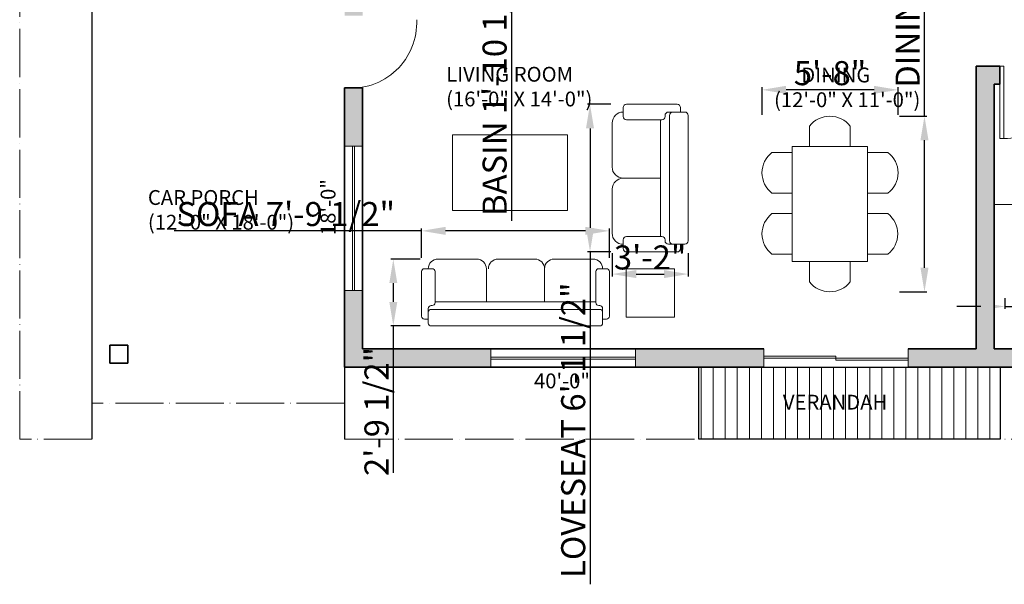
# Model space of a CAD drawing. Units: inches. Extents: x 2364 to 7426, y 1289 to 11972.
# Tile 1 of 6: x 2432 to 2923, y 1289 to 1571. Entities that reach past the tile are written whole.
import ezdxf

# ---------------------------------------------------------------- set-up
doc = ezdxf.new("R2010")
doc.units = ezdxf.units.IN
doc.linetypes.add('ACAD_ISO04W100', pattern=[30, 24, -3, 0, -3])
for name, color, linetype, lineweight in [('A-ANNO-DIMS', 2, 'Continuous', 15), ('A-AREA-IDEN', 7, 'Continuous', 18), ('A-COLS', 7, 'Continuous', 35), ('A-DOOR', 3, 'Continuous', 18), ('A-FLOR', 7, 'Continuous', 25), ('A-FLOR-CASE', 8, 'Continuous', 18), ('A-FLOR-PATT', 9, 'Continuous', 13), ('A-FURN', 8, 'Continuous', 15), ('A-GLAZ', 4, 'Continuous', 18), ('A-WALL', 7, 'Continuous', 35), ('C-PROP', 3, 'ACAD_ISO04W100', 18)]:
    doc.layers.add(name, color=color, linetype=linetype, lineweight=lineweight)
doc.layers.add('A-WALL-PATT', color=251, linetype='Continuous', lineweight=13, true_color=0x636466)
doc.styles.get("Standard").update_dxf_attribs({"font": 'arial.ttf'})
doc.dimstyles.new('ISO-25', dxfattribs={"dimtxt": 12, "dimasz": 12, "dimexe": 1.25, "dimexo": 0.625, "dimtad": 1, "dimlunit": 3, "dimtxsty": 'Standard', "dimcen": 2.5, "dimadec": 0, "dimazin": 0, "dimtfac": 1, "dimtmove": 0, "dimatfit": 3, "dimfxl": 1, "dimarcsym": 0})

# ---------------------------------------------------------------- blocks, each defined once
blk = doc.blocks.new('DINING TABLE')
for p, q in [((2443.51, 1632.65), (2443.51, 1644.65)), ((2467.51, 1632.65), (2467.51, 1644.65)), ((2479.51, 1632.65), (2479.51, 1644.65)), ((2503.51, 1632.65), (2503.51, 1644.65)), ((2427.28, 1622.52), (2439.28, 1622.52)), ((2507.03, 1622.52), (2519.03, 1622.52)), ((2427.28, 1598.52), (2439.28, 1598.52)), ((2507.03, 1598.52), (2519.03, 1598.52)), ((2443.51, 1576.39), (2443.51, 1588.39)), ((2467.51, 1576.39), (2467.51, 1588.39)), ((2479.51, 1576.39), (2479.51, 1588.39)), ((2503.51, 1576.39), (2503.51, 1588.39))]:
    blk.add_line(p, q)
blk.add_lwpolyline([(2439.28, 1632.65), (2507.03, 1632.65), (2507.03, 1588.39), (2439.28, 1588.39)], close=True)
for centre, radius, start, end in [((2455.51, 1635.3), 15.21, 37.93078, 142.06922), ((2491.51, 1635.3), 15.21, 37.93078, 142.06922), ((2436.64, 1610.52), 15.21, 127.93078, 232.06922), ((2509.67, 1610.52), 15.21, 307.93078, 52.06922), ((2455.51, 1585.74), 15.21, 217.93078, 322.06922), ((2491.51, 1585.15), 14.86, 216.12624, 323.87376)]:
    blk.add_arc(centre, radius, start, end)
blk = doc.blocks.new('A$C115861F8')
for p, q in [((0.0679, 0.6013), (0.0291, 0.6013)), ((0.0679, 0.6401), (0.0679, 0.6013)), ((0.0679, 0.5334), (0.0679, 0.6013)), ((1.7846, 0.6692), (0.097, 0.6692)), ((1.8136, 0.6401), (1.8136, 0.6013)), ((1.8136, 0.6013), (1.8524, 0.6013)), ((1.8136, 0.5334), (1.8136, 0.6013)), ((0, 0.5722), (0, 0.1261)), ((0.0679, 0.4946), (0.0679, 0.5431)), ((1.7846, 0.5043), (0.097, 0.5043)), ((1.8136, 0.4946), (1.8136, 0.5431)), ((1.8815, 0.5722), (1.8815, 0.1261)), ((0.1067, 0.4655), (0.097, 0.4655)), ((0.1358, 0.1261), (0.1358, 0.4364)), ((1.7458, 0.4267), (0.1358, 0.4267)), ((0.6498, 0.097), (0.6498, 0.4267)), ((1.2317, 0.097), (1.2317, 0.4267)), ((1.7458, 0.1261), (1.7458, 0.4364)), ((1.7749, 0.4655), (1.7846, 0.4655)), ((0.0291, 0.097), (0.1067, 0.097)), ((0.1649, 0), (0.5528, 0)), ((1.1347, 0), (0.7468, 0)), ((1.3287, 0), (1.7167, 0)), ((1.8524, 0.097), (1.7749, 0.097))]:
    blk.add_line(p, q)
for centre, radius, start, end in [((0.0291, 0.5722), 0.0291, 90, 180), ((0.097, 0.6401), 0.0291, 90, 180), ((1.7846, 0.6401), 0.0291, 0, 90), ((1.8524, 0.5722), 0.0291, 0, 90), ((0.097, 0.5334), 0.0291, 180, 270), ((0.097, 0.4946), 0.0291, 180, 270), ((1.7846, 0.5334), 0.0291, 270, 0), ((1.7846, 0.4946), 0.0291, 270, 0), ((0.1067, 0.4364), 0.0291, 0, 90), ((1.7749, 0.4364), 0.0291, 90, 180), ((0.0291, 0.1261), 0.0291, 180, 270), ((0.1067, 0.1261), 0.0291, 270, 0), ((1.7749, 0.1261), 0.0291, 180, 270), ((1.8524, 0.1261), 0.0291, 270, 0), ((0.1649, 0.097), 0.097, 180, 270), ((0.5528, 0.097), 0.097, 270, 0), ((0.7468, 0.097), 0.097, 180, 270), ((1.1147, 0.097), 0.097, 270, 0), ((1.3287, 0.097), 0.097, 180, 270), ((1.7167, 0.097), 0.097, 270, 0)]:
    blk.add_arc(centre, radius, start, end)
blk = doc.blocks.new('A$C02A636C4')
for p, q in [((0.0679, 0.6401), (0.0679, 0.6013)), ((1.2026, 0.6692), (0.097, 0.6692)), ((1.2317, 0.6401), (1.2317, 0.6013)), ((0, 0.5722), (0, 0.1261)), ((0.0679, 0.6013), (0.0291, 0.6013)), ((0.0679, 0.5334), (0.0679, 0.6013)), ((0.0679, 0.4946), (0.0679, 0.5431)), ((1.2317, 0.6013), (1.2705, 0.6013)), ((1.2317, 0.5334), (1.2317, 0.6013)), ((1.2317, 0.4946), (1.2317, 0.5431)), ((1.2996, 0.5722), (1.2996, 0.1261)), ((1.2026, 0.5043), (0.097, 0.5043)), ((0.1067, 0.4655), (0.097, 0.4655)), ((0.1358, 0.1261), (0.1358, 0.4364)), ((1.1638, 0.1261), (1.1638, 0.4364)), ((1.1929, 0.4655), (1.2026, 0.4655)), ((1.1638, 0.4267), (0.1358, 0.4267)), ((0.6498, 0.097), (0.6498, 0.4267)), ((0.0291, 0.097), (0.1067, 0.097)), ((1.2705, 0.097), (1.1929, 0.097)), ((0.1649, 0), (0.5528, 0)), ((0.7468, 0), (1.1347, 0))]:
    blk.add_line(p, q)
for centre, radius, start, end in [((0.097, 0.6401), 0.0291, 90, 180), ((1.2026, 0.6401), 0.0291, 0, 90), ((0.0291, 0.5722), 0.0291, 90, 180), ((0.097, 0.5334), 0.0291, 180, 270), ((1.2026, 0.5334), 0.0291, 270, 0), ((1.2705, 0.5722), 0.0291, 0, 90), ((0.097, 0.4946), 0.0291, 180, 270), ((0.1067, 0.4364), 0.0291, 0, 90), ((1.1929, 0.4364), 0.0291, 90, 180), ((1.2026, 0.4946), 0.0291, 270, 0), ((0.0291, 0.1261), 0.0291, 180, 270), ((0.1649, 0.097), 0.097, 180, 270), ((0.1067, 0.1261), 0.0291, 270, 0), ((0.5528, 0.097), 0.097, 270, 0), ((0.7468, 0.097), 0.097, 180, 270), ((1.1347, 0.097), 0.097, 270, 0), ((1.1929, 0.1261), 0.0291, 180, 270), ((1.2705, 0.1261), 0.0291, 270, 0)]:
    blk.add_arc(centre, radius, start, end)
blk = doc.blocks.new('WIN-72IN')
for p, q in [((0, 0), (0, 9)), ((72, 5), (0, 5)), ((72, 0), (72, 9)), ((72, 4), (0, 4))]:
    blk.add_line(p, q)
blk = doc.blocks.new('SIDE-TABLE-24IN')
blk.add_lwpolyline([(24, 24), (24, 0), (0, 0), (0, 24)], close=True)
blk = doc.blocks.new('*D39')
at = {"layer": 'A-ANNO-DIMS', "color": 0, "lineweight": -2, "transparency": 16777216}
for p, q in [((2677.33, 1695.23), (2677.33, 1707.23)), ((2680.1, 1683.23), (2676.08, 1683.23)), ((2677.33, 1683.23), (2677.33, 1660.64)), ((2680.1, 1660.64), (2676.08, 1660.64)), ((2677.33, 1648.64), (2677.33, 1470.52))]:
    blk.add_line(p, q, dxfattribs=at)
at = {"layer": 'A-ANNO-DIMS', "color": 0, "lineweight": 100, "transparency": 16777216}
for points in [[(2675.33, 1695.23), (2679.33, 1695.23), (2677.33, 1683.23)], [(2675.33, 1648.64), (2679.33, 1648.64), (2677.33, 1660.64)]]:
    blk.add_solid(points, dxfattribs=at)
at = {"layer": 'Defpoints', "color": 0, "lineweight": 100, "transparency": 16777216}
for p in [(2680.72, 1683.23), (2677.33, 1660.64), (2680.72, 1660.64)]:
    blk.add_point(p, dxfattribs=at)
at = {"layer": 'A-ANNO-DIMS', "color": 0, "transparency": 16777216, "insert": (2670.5, 1553.58), "char_height": 12, "attachment_point": 5, "rotation": 90}
blk.add_mtext('BASIN 1\'-10 1/2" TYP.', dxfattribs=at)
blk = doc.blocks.new('*D41')
at = {"layer": 'A-ANNO-DIMS', "color": 0, "lineweight": -2, "transparency": 16777216}
for p, q in [((2883.34, 1522.66), (2883.34, 1695.76)), ((2870.82, 1522.66), (2884.59, 1522.66)), ((2883.34, 1447.09), (2883.34, 1510.66)), ((2870.82, 1435.09), (2884.59, 1435.09))]:
    blk.add_line(p, q, dxfattribs=at)
at = {"layer": 'A-ANNO-DIMS', "color": 0, "lineweight": 100, "transparency": 16777216}
for points in [[(2881.34, 1510.66), (2885.34, 1510.66), (2883.34, 1522.66)], [(2881.34, 1447.09), (2885.34, 1447.09), (2883.34, 1435.09)]]:
    blk.add_solid(points, dxfattribs=at)
at = {"layer": 'Defpoints', "color": 0, "lineweight": 100, "transparency": 16777216}
for p in [(2870.2, 1522.66), (2883.34, 1522.66), (2870.2, 1435.09)]:
    blk.add_point(p, dxfattribs=at)
at = {"layer": 'A-ANNO-DIMS', "color": 0, "transparency": 16777216, "insert": (2876.5, 1615.21), "char_height": 12, "attachment_point": 5, "rotation": 90}
blk.add_mtext('DINING SET 7\'-3 1/2"', dxfattribs=at)
blk = doc.blocks.new('*D42')
at = {"layer": 'A-ANNO-DIMS', "color": 0, "lineweight": -2, "transparency": 16777216}
for p, q in [((2802.31, 1523.28), (2802.31, 1537.04)), ((2870.2, 1523.28), (2870.2, 1537.04)), ((2858.2, 1535.79), (2814.31, 1535.79))]:
    blk.add_line(p, q, dxfattribs=at)
at = {"layer": 'A-ANNO-DIMS', "color": 0, "lineweight": 100, "transparency": 16777216}
for points in [[(2814.31, 1537.79), (2814.31, 1533.79), (2802.31, 1535.79)], [(2858.2, 1537.79), (2858.2, 1533.79), (2870.2, 1535.79)]]:
    blk.add_solid(points, dxfattribs=at)
at = {"layer": 'Defpoints', "color": 0, "lineweight": 100, "transparency": 16777216}
for p in [(2802.31, 1535.79), (2802.31, 1522.66), (2870.2, 1522.66)]:
    blk.add_point(p, dxfattribs=at)
at = {"layer": 'A-ANNO-DIMS', "color": 0, "transparency": 16777216, "insert": (2836.25, 1542.55), "char_height": 12, "attachment_point": 5}
blk.add_mtext('5\'-8"', dxfattribs=at)
blk = doc.blocks.new('*D43')
at = {"layer": 'A-ANNO-DIMS', "color": 0, "lineweight": -2, "transparency": 16777216}
for p, q in [((2632.49, 1465.45), (2509.14, 1465.45)), ((2632.49, 1452.02), (2632.49, 1466.7)), ((2714.22, 1465.45), (2644.49, 1465.45)), ((2726.22, 1452.02), (2726.22, 1466.7))]:
    blk.add_line(p, q, dxfattribs=at)
at = {"layer": 'A-ANNO-DIMS', "color": 0, "lineweight": 100, "transparency": 16777216}
for points in [[(2644.49, 1467.45), (2644.49, 1463.45), (2632.49, 1465.45)], [(2714.22, 1467.45), (2714.22, 1463.45), (2726.22, 1465.45)]]:
    blk.add_solid(points, dxfattribs=at)
at = {"layer": 'Defpoints', "color": 0, "lineweight": 100, "transparency": 16777216}
for p in [(2632.49, 1465.45), (2632.49, 1451.39), (2726.22, 1451.39)]:
    blk.add_point(p, dxfattribs=at)
at = {"layer": 'A-ANNO-DIMS', "color": 0, "transparency": 16777216, "insert": (2564.81, 1472.29), "char_height": 12, "attachment_point": 5}
blk.add_mtext('SOFA 7\'-9 1/2"', dxfattribs=at)
blk = doc.blocks.new('*D44')
at = {"layer": 'A-ANNO-DIMS', "color": 0, "lineweight": -2, "transparency": 16777216}
for p, q in [((2631.86, 1451.39), (2617.18, 1451.39)), ((2618.43, 1439.39), (2618.43, 1430.06)), ((2631.86, 1418.06), (2617.18, 1418.06)), ((2618.43, 1418.06), (2618.43, 1344.74))]:
    blk.add_line(p, q, dxfattribs=at)
at = {"layer": 'A-ANNO-DIMS', "color": 0, "lineweight": 100, "transparency": 16777216}
for points in [[(2616.43, 1439.39), (2620.43, 1439.39), (2618.43, 1451.39)], [(2616.43, 1430.06), (2620.43, 1430.06), (2618.43, 1418.06)]]:
    blk.add_solid(points, dxfattribs=at)
at = {"layer": 'Defpoints', "color": 0, "lineweight": 100, "transparency": 16777216}
for p in [(2632.49, 1451.39), (2618.43, 1418.06), (2632.49, 1418.06)]:
    blk.add_point(p, dxfattribs=at)
at = {"layer": 'A-ANNO-DIMS', "color": 0, "transparency": 16777216, "insert": (2611.6, 1375.4), "char_height": 12, "attachment_point": 5, "rotation": 90}
blk.add_mtext('2\'-9 1/2"', dxfattribs=at)
blk = doc.blocks.new('*D45')
at = {"layer": 'A-ANNO-DIMS', "color": 0, "lineweight": -2, "transparency": 16777216}
for p, q in [((2726.96, 1528.56), (2715.29, 1528.56)), ((2716.54, 1516.56), (2716.54, 1466.93)), ((2726.96, 1454.93), (2715.29, 1454.93)), ((2716.54, 1454.93), (2716.54, 1289.19))]:
    blk.add_line(p, q, dxfattribs=at)
at = {"layer": 'A-ANNO-DIMS', "color": 0, "lineweight": 100, "transparency": 16777216}
for points in [[(2714.54, 1516.56), (2718.54, 1516.56), (2716.54, 1528.56)], [(2714.54, 1466.93), (2718.54, 1466.93), (2716.54, 1454.93)]]:
    blk.add_solid(points, dxfattribs=at)
at = {"layer": 'Defpoints', "color": 0, "lineweight": 100, "transparency": 16777216}
for p in [(2727.58, 1528.56), (2716.54, 1454.93), (2727.58, 1454.93)]:
    blk.add_point(p, dxfattribs=at)
at = {"layer": 'A-ANNO-DIMS', "color": 0, "transparency": 16777216, "insert": (2709.7, 1366.06), "char_height": 12, "attachment_point": 5, "rotation": 90}
blk.add_mtext('LOVESEAT 6\'-1 1/2"', dxfattribs=at)
blk = doc.blocks.new('*D46')
at = {"layer": 'A-ANNO-DIMS', "color": 0, "lineweight": -2, "transparency": 16777216}
for p, q in [((2727.58, 1454.31), (2727.58, 1442.64)), ((2765.49, 1454.31), (2765.49, 1442.64)), ((2739.58, 1443.89), (2753.49, 1443.89))]:
    blk.add_line(p, q, dxfattribs=at)
at = {"layer": 'A-ANNO-DIMS', "color": 0, "lineweight": 100, "transparency": 16777216}
for points in [[(2739.58, 1445.89), (2739.58, 1441.89), (2727.58, 1443.89)], [(2753.49, 1445.89), (2753.49, 1441.89), (2765.49, 1443.89)]]:
    blk.add_solid(points, dxfattribs=at)
at = {"layer": 'Defpoints', "color": 0, "lineweight": 100, "transparency": 16777216}
for p in [(2727.58, 1454.93), (2765.49, 1454.93), (2765.49, 1443.89)]:
    blk.add_point(p, dxfattribs=at)
at = {"layer": 'A-ANNO-DIMS', "color": 0, "transparency": 16777216, "insert": (2746.54, 1450.65), "char_height": 12, "attachment_point": 5}
blk.add_mtext('3\'-2"', dxfattribs=at)
blk = doc.blocks.new('*D51')
at = {"layer": 'A-ANNO-DIMS', "color": 0, "lineweight": -2, "transparency": 16777216}
for p, q in [((2951.87, 1464.26), (2951.87, 1625.72)), ((2947.73, 1464.26), (2953.12, 1464.26)), ((2951.87, 1444.52), (2951.87, 1452.26)), ((2947.73, 1432.52), (2953.12, 1432.52))]:
    blk.add_line(p, q, dxfattribs=at)
at = {"layer": 'A-ANNO-DIMS', "color": 0, "lineweight": 100, "transparency": 16777216}
for points in [[(2949.87, 1452.26), (2953.87, 1452.26), (2951.87, 1464.26)], [(2949.87, 1444.52), (2953.87, 1444.52), (2951.87, 1432.52)]]:
    blk.add_solid(points, dxfattribs=at)
at = {"layer": 'Defpoints', "color": 0, "lineweight": 100, "transparency": 16777216}
for p in [(2947.11, 1464.26), (2951.87, 1464.26), (2947.11, 1432.52)]:
    blk.add_point(p, dxfattribs=at)
at = {"layer": 'A-ANNO-DIMS', "color": 0, "transparency": 16777216, "insert": (2945.04, 1550.99), "char_height": 12, "attachment_point": 5, "rotation": 90}
blk.add_mtext('COOKTOP 2\'-7 1/2"', dxfattribs=at)
blk = doc.blocks.new('*D52')
at = {"layer": 'A-ANNO-DIMS', "color": 0, "lineweight": -2, "transparency": 16777216}
for p, q in [((2923.4, 1431.9), (2923.4, 1426.51)), ((2947.11, 1431.9), (2947.11, 1426.51)), ((2911.4, 1427.76), (2899.4, 1427.76)), ((2923.4, 1427.76), (2947.11, 1427.76)), ((2959.11, 1427.76), (3040.41, 1427.76))]:
    blk.add_line(p, q, dxfattribs=at)
at = {"layer": 'A-ANNO-DIMS', "color": 0, "lineweight": 100, "transparency": 16777216}
for points in [[(2911.4, 1429.76), (2911.4, 1425.76), (2923.4, 1427.76)], [(2959.11, 1429.76), (2959.11, 1425.76), (2947.11, 1427.76)]]:
    blk.add_solid(points, dxfattribs=at)
at = {"layer": 'Defpoints', "color": 0, "lineweight": 100, "transparency": 16777216}
for p in [(2923.4, 1432.52), (2947.11, 1432.52), (2947.11, 1427.76)]:
    blk.add_point(p, dxfattribs=at)
at = {"layer": 'A-ANNO-DIMS', "color": 0, "transparency": 16777216, "insert": (3005.76, 1434.59), "char_height": 12, "attachment_point": 5}
blk.add_mtext('1\'-11 1/2"', dxfattribs=at)

msp = doc.modelspace()

# ---------------------------------------------------------------- hatches: boundary and pattern name
at = {"layer": 'A-FLOR-PATT'}
h = msp.add_hatch(dxfattribs=at)
h.set_pattern_fill('ANSI31', color=256, scale=1.889764, angle=45, style=0)
h.paths.add_polyline_path([(2770.735, 1361.544), (2921.103, 1361.544), (2921.103, 1397.544), (2770.735, 1397.544)])
at = {"layer": 'A-WALL-PATT'}
h = msp.add_hatch(color=256, dxfattribs=at)
h.dxf.hatch_style = 1
h.paths.add_polyline_path([(2522.103, 1763.544), (2477.103, 1763.544), (2477.103, 1646.544), (2486.103, 1646.544), (2486.103, 1754.544), (2522.103, 1754.544)])
h.paths.add_polyline_path([(2657.103, 1763.544), (2594.103, 1763.544), (2594.103, 1754.544), (2630.103, 1754.544), (2630.103, 1625.388), (2632.457, 1625.388, -0.0509344), (2639.103, 1625.388), (2639.103, 1654.044), (2640.627, 1654.044), (2640.627, 1658.544), (2639.103, 1658.544), (2639.103, 1754.544), (2657.103, 1754.544)])
h.paths.add_polyline_path([(2746.353, 1763.544), (2681.103, 1763.544), (2681.103, 1754.544), (2699.103, 1754.544), (2699.103, 1658.544), (2670.627, 1658.544), (2670.627, 1656.552, -0.0218135), (2670.627, 1654.044), (2699.103, 1654.044), (2699.103, 1595.544), (2820.603, 1595.544, -0.0518861), (2820.603, 1602.304), (2820.603, 1604.544), (2708.103, 1604.544), (2708.103, 1754.544), (2746.353, 1754.544)])
h.paths.add_polyline_path([(2879.103, 1763.544), (2818.353, 1763.544), (2818.353, 1754.544), (2856.603, 1754.544), (2856.603, 1666.044), (2921.103, 1666.044), (2921.103, 1604.544), (2897.103, 1604.544), (2897.103, 1595.544), (2930.103, 1595.544), (2930.103, 1627.044), (2930.103, 1754.544), (3062.103, 1754.544), (3062.103, 1715.544), (3071.103, 1715.544), (3071.103, 1763.544), (2903.103, 1763.544), (2903.103, 1754.544), (2921.103, 1754.544), (2921.103, 1670.544), (2861.103, 1670.544), (2861.103, 1754.544), (2879.103, 1754.544)])
h.paths.add_polyline_path([(3071.103, 1643.544), (3062.103, 1643.544), (3062.103, 1604.544), (2961.603, 1604.544), (2961.603, 1601.334, -0.0507006), (2961.603, 1595.544), (2961.603, 1574.085, -0.036481), (2964.864, 1574.085), (2966.103, 1574.085), (2966.103, 1595.544), (3062.103, 1595.544), (3062.103, 1583.544), (3071.103, 1583.544)])
h.paths.add_polyline_path([(3071.103, 1559.544), (3062.103, 1559.544), (3062.103, 1547.544), (2966.103, 1547.544), (2966.103, 1550.085), (2961.603, 1550.085), (2961.603, 1547.544), (2956.9, 1547.544, -0.039283), (2956.9, 1542.306), (2956.9, 1538.544), (3062.103, 1538.544), (3062.103, 1508.544), (3071.103, 1508.544)])
h.paths.add_polyline_path([(3071.103, 1436.544), (3062.103, 1436.544), (3062.103, 1406.544), (3020.103, 1406.544), (3020.103, 1397.544), (3071.103, 1397.544)])
h.paths.add_polyline_path([(2960.103, 1406.544), (2918.103, 1406.544), (2918.103, 1538.544), (2920.9, 1538.544), (2920.9, 1547.544), (2909.103, 1547.544), (2909.103, 1406.544), (2875.194, 1406.544), (2875.194, 1397.544), (2921.103, 1397.544), (2960.103, 1397.544)])
h.paths.add_polyline_path([(2803.194, 1406.544), (2739.149, 1406.544), (2739.149, 1397.544), (2803.194, 1397.544)])
h.paths.add_polyline_path([(2667.149, 1406.544), (2603.103, 1406.544), (2603.103, 1435.657), (2594.103, 1435.657), (2594.103, 1397.544), (2667.149, 1397.544)])
h.paths.add_polyline_path([(2603.103, 1536.771), (2600.612, 1536.771, -0.0497705), (2594.103, 1536.771), (2594.103, 1507.657), (2603.103, 1507.657)])
h.paths.add_polyline_path([(2639.103, 1589.388), (2630.103, 1589.388), (2630.103, 1586.544), (2486.103, 1586.544), (2486.103, 1610.544), (2477.103, 1610.544), (2477.103, 1577.544), (2594.103, 1577.544), (2594.103, 1572.771), (2603.103, 1572.771), (2603.103, 1577.544), (2639.103, 1577.544)])
h.paths.add_polyline_path([(2636.627, 1719.186), (2701.024, 1719.186), (2701.024, 1746.896), (2636.627, 1746.896)], flags=9)

# ---------------------------------------------------------------- linework, layer by layer
at = {"layer": 'A-COLS'}
for p, q in [((2477.103, 1408.405), (2477.103, 1399.405)), ((2477.103, 1408.405), (2486.103, 1408.405)), ((2486.103, 1408.405), (2486.103, 1399.405)), ((2477.103, 1399.405), (2486.103, 1399.405))]:
    msp.add_line(p, q, dxfattribs=at)
at = {"layer": 'A-DOOR'}
for p, q in [((2920.9, 1547.544), (2920.9, 1511.544)), ((2922.9, 1547.544), (2920.9, 1547.544)), ((2922.9, 1511.544), (2922.9, 1547.544)), ((2920.9, 1511.544), (2922.9, 1511.544)), ((2803.194, 1406.544), (2803.194, 1397.544)), ((2875.194, 1406.544), (2875.194, 1397.544)), ((2803.194, 1403.044), (2839.194, 1403.044)), ((2803.194, 1402.044), (2875.194, 1402.044)), ((2839.194, 1403.044), (2839.194, 1401.044)), ((2839.194, 1401.044), (2875.194, 1401.044))]:
    msp.add_line(p, q, dxfattribs=at)
for centre, radius, start, end in [((2597.358, 1569.384), 32.775, 264.30142, 2.42543), ((2923.614, 1544.925), 33.388, 268.77397, 4.49919)]:
    msp.add_arc(centre, radius, start, end, dxfattribs=at)
at = {"layer": 'A-FLOR'}
for p, q in [((2468.103, 1577.544), (2468.103, 1361.544)), ((2594.103, 1397.544), (2594.103, 1361.544)), ((2770.735, 1361.544), (2770.735, 1397.544)), ((2803.194, 1397.544), (2875.194, 1397.544)), ((2921.103, 1397.544), (2921.103, 1361.544)), ((2921.103, 1361.544), (2770.735, 1361.544))]:
    msp.add_line(p, q, dxfattribs=at)
at = {"layer": 'A-FLOR-CASE'}
msp.add_line((2954.103, 1478.544), (2918.103, 1478.544), dxfattribs=at)
at = {"layer": 'A-FURN'}
msp.add_lwpolyline([(2647.922, 1513.389), (2705.264, 1513.389), (2705.264, 1475.605), (2647.922, 1475.605)], close=True, dxfattribs=at)
at = {"layer": 'A-WALL'}
for p, q in [((2909.103, 1547.544), (2920.9, 1547.544)), ((2909.103, 1406.544), (2909.103, 1547.544)), ((2920.9, 1538.544), (2920.9, 1547.544)), ((2918.103, 1538.544), (2920.9, 1538.544)), ((2918.103, 1406.544), (2918.103, 1538.544)), ((2594.103, 1397.544), (2594.103, 1536.771)), ((2594.103, 1536.771), (2603.103, 1536.771)), ((2603.103, 1406.544), (2603.103, 1536.771)), ((2603.103, 1406.544), (2803.194, 1406.544)), ((2875.194, 1406.544), (2909.103, 1406.544)), ((2918.103, 1406.544), (3062.103, 1406.544)), ((2803.194, 1397.544), (2594.103, 1397.544)), ((2921.103, 1397.544), (2875.194, 1397.544)), ((2921.103, 1397.544), (3071.103, 1397.544))]:
    msp.add_line(p, q, dxfattribs=at)
at = {"layer": 'C-PROP'}
for p, q in [((2432.103, 1361.544), (2432.103, 1791.071)), ((2594.103, 1379.544), (2468.103, 1379.544)), ((2468.103, 1361.544), (2432.103, 1361.544)), ((2594.103, 1361.544), (2770.735, 1361.544)), ((3131.103, 1361.544), (2921.103, 1361.544))]:
    msp.add_line(p, q, dxfattribs=at)

# ---------------------------------------------------------------- block references
at = {"layer": 'A-FURN'}
for name, p, xscale, yscale, zscale, rotation in [('A$C02A636C4', (2727.58, 1528.564), 56.65455893346969, 56.65455893346969, 56.65455893346969, 270), ('DINING TABLE', (4199.258, -614.346), 0.8463755954016345, 0.8463755954016345, 0.8463755954016345, 90), ('A$C115861F8', (2726.222, 1451.394), 49.81716244564395, 49.81716244564395, 49.81716244564395, 180.0000000000008)]:
    msp.add_blockref(name, p, dxfattribs=dict(at, xscale=xscale, yscale=yscale, zscale=zscale, rotation=rotation))
msp.add_blockref('SIDE-TABLE-24IN', (2734.623, 1422.492), dxfattribs=at)
at = {"layer": 'A-GLAZ'}
for p, rotation in [((2594.103, 1507.657), 270), ((2739.149, 1406.544), 180)]:
    msp.add_blockref('WIN-72IN', p, dxfattribs=dict(at, rotation=rotation))

# ---------------------------------------------------------------- texts
at = {"layer": 'A-ANNO-DIMS', "insert": (2582.206, 1463.375), "char_height": 7.4003, "attachment_point": 1, "rotation": 90}
msp.add_mtext_dynamic_manual_height_columns('18\'-0"', width=192.6715, gutter_width=37.001, heights=[0], dxfattribs=at)
at = {"layer": 'A-ANNO-DIMS', "insert": (2688.601, 1394.328), "char_height": 7.4003, "attachment_point": 1}
msp.add_mtext_dynamic_manual_height_columns('40\'-0"', width=192.6715, gutter_width=37.001, heights=[0], dxfattribs=at)
at = {"layer": 'A-AREA-IDEN', "attachment_point": 1}
for s, insert, char_height in [('LIVING ROOM \\P(16\'-0" X 14\'-0")', (2644.782, 1547.258), 7.40027), ('      DINING\\P(12\'-0" X 11\'-0")', (2808.323, 1546.885), 7.40027), ('CAR PORCH\\P(12\'-0" X 18\'-0")', (2496.043, 1485.798), 7.40027), ('VERANDAH', (2812.735, 1383.712), 7.4003)]:
    msp.add_mtext_dynamic_manual_height_columns(s, width=192.6715, gutter_width=37.001, heights=[0], dxfattribs=dict(at, insert=insert, char_height=char_height))

# ---------------------------------------------------------------- dimensions: what is measured, and where the dimension line sits
at = {"layer": 'A-ANNO-DIMS'}
for base, p1, p2, angle, text, picture, middle in [((2677.334, 1660.636), (2680.723, 1683.228), (2680.723, 1660.636), 270, 'BASIN <> TYP.', '*D39', (2670.504, 1553.578)), ((2883.336, 1522.658), (2870.2, 1435.086), (2870.2, 1522.658), 90, 'DINING SET <>', '*D41', (2876.502, 1615.21)), ((2951.87, 1464.259), (2947.11, 1432.522), (2947.11, 1464.259), 90, 'COOKTOP <>', '*D51', (2945.037, 1550.988)), ((2716.536, 1454.934), (2727.58, 1528.564), (2727.58, 1454.934), 270, 'LOVESEAT <>', '*D45', (2709.702, 1366.061)), ((2632.489, 1465.454), (2726.222, 1451.394), (2632.489, 1451.394), 180, 'SOFA <>', '*D43', (2564.812, 1472.288))]:
    dim = msp.add_linear_dim(base=base, p1=p1, p2=p2, angle=angle, text=text, dimstyle='ISO-25', override={"dimdec": 1, "dimlfac": 1, "dimrnd": 0, "dimzin": 1, "dimdsep": 46, "dimlunit": 4, "dimfrac": 2}, dxfattribs=at)
    dim.commit()
    dim.dimension.update_dxf_attribs({"geometry": picture, "text_midpoint": middle})
for base, p1, p2, angle, picture, middle in [((2802.307, 1535.793), (2870.2, 1522.658), (2802.307, 1522.658), 180, '*D42', (2836.253, 1542.545)), ((2618.429, 1418.056), (2632.489, 1451.394), (2632.489, 1418.056), 270, '*D44', (2611.599, 1375.398))]:
    dim = msp.add_linear_dim(base=base, p1=p1, p2=p2, angle=angle, dimstyle='ISO-25', override={"dimdec": 1, "dimlfac": 1, "dimrnd": 0, "dimzin": 1, "dimdsep": 46, "dimlunit": 4, "dimfrac": 2}, dxfattribs=at)
    dim.commit()
    dim.dimension.update_dxf_attribs({"geometry": picture, "text_midpoint": middle})
for base, p1, p2, picture, middle in [((2765.494, 1443.89), (2727.58, 1454.934), (2765.494, 1454.934), '*D46', (2746.537, 1450.646)), ((2947.11, 1427.761), (2923.405, 1432.522), (2947.11, 1432.522), '*D52', (3005.762, 1434.591))]:
    dim = msp.add_linear_dim(base=base, p1=p1, p2=p2, dimstyle='ISO-25', override={"dimdec": 1, "dimlfac": 1, "dimrnd": 0, "dimzin": 1, "dimdsep": 46, "dimlunit": 4, "dimfrac": 2}, dxfattribs=at)
    dim.commit()
    dim.dimension.update_dxf_attribs({"geometry": picture, "text_midpoint": middle})

doc.saveas('drawing.dxf')
